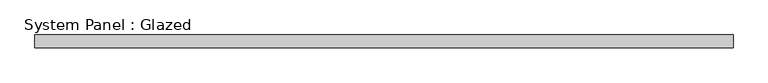
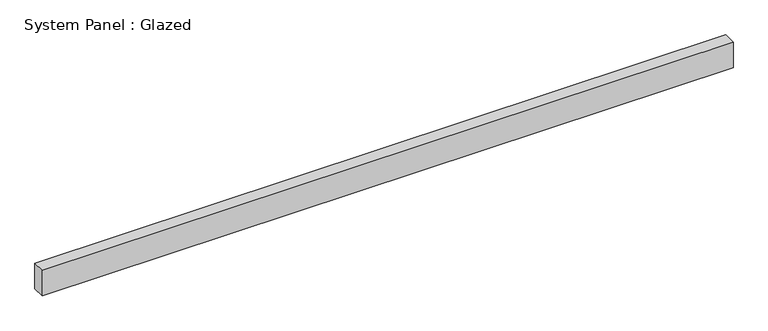
"""IFC4 building model written with IfcOpenShell, lengths in millimetres: plate geometry, System Panel : Glazed."""

from ifc_helpers import new_model, si_unit, origin, origin_with_axes, place, context, project, spatial, polyline, outline, extrude, source, transform, mapped, element, save


def system_panel_glazed_a1658219(model_context):
    return source(origin(), model_context, "Body", "SweptSolid", [
        extrude(outline(polyline([(688.9750001, 19.05), (-688.9750001, 19.05), (-688.9750001, 44.45), (688.9750001, 44.45), (688.9750001, 19.05)])), origin_with_axes(), (0.0, 0.0, 1.0), 53.5691055),
    ])


if __name__ == "__main__":
    model = new_model("IFC4")
    model_context = context("Model", 3, world=origin())
    ifc_project = project(units=[si_unit("LENGTHUNIT", "METRE", prefix="MILLI")], contexts=[model_context])
    site = spatial("IfcSite", under=ifc_project)
    building = spatial("IfcBuilding", under=site)
    placement = place(None, origin())
    system_panel_glazed_shape = system_panel_glazed_a1658219(model_context)
    element("IfcPlate", 1, ObjectType="System Panel : Glazed", at=placement, inside=building, context=model_context, shape_type="MappedRepresentation", body=[
        mapped(system_panel_glazed_shape, transform((0.0, 0.0, 0.0), x_axis=(1.0, 0.0, 0.0), y_axis=(0.0, 1.0, 0.0), z_axis=(0.0, 0.0, 1.0))),
    ])
    save(model, "model.ifc")

# Revit data of these elements
# Type "System Panel : Glazed"
#   Construction Type Id = "GSP4R"
#   Analytic Construction = "1/8 in Pilkington single glazing"
#   Visual Light Transmittance = 0.9
#   Solar Heat Gain Coefficient = 0.86
#   Heat Transfer Coefficient (U) = 1.18115 BTU/(h·ft²·°F)
#   Define Thermal Properties by = 1
# Element 1 (IfcPlate, "System Panel : Glazed")
#   Materials on its faces: "Glass"
# Materials
#   "Glass": class "Glass", colour RGB 0 128 192, transparency 0.75, Description = "Soda Lime Glass", Cost = 0
